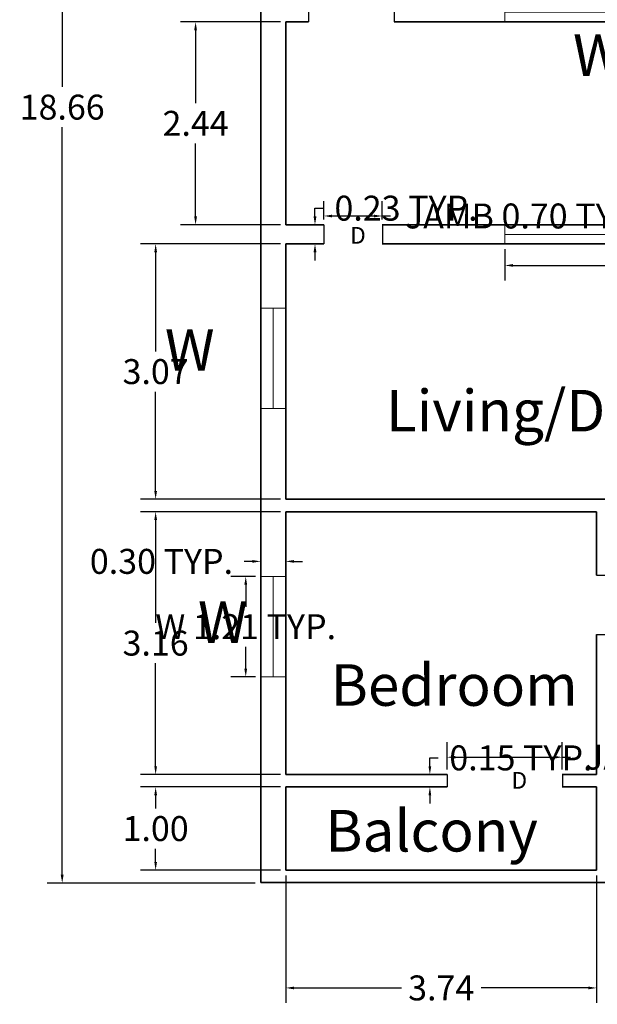
# Model space of a CAD drawing. Units: metres. Extents: x 11 to 49.6, y -23.3 to -0.8.
# Tile 1 of 5: x 11 to 17.9, y -23.3 to -11.5. Entities that reach past the tile are written whole.
import ezdxf

# ---------------------------------------------------------------- set-up
doc = ezdxf.new("R2010")
doc.units = ezdxf.units.M
doc.header["$MEASUREMENT"] = 0
for name, color, linetype, lineweight in [('A-ANNO-DIMS', 2, 'Continuous', 18), ('A-ANNO-IDEN', 3, 'Continuous', 18), ('A-AREA-IDEN', 7, 'Continuous', 18), ('A-DOOR', 3, 'Continuous', 25), ('A-GLAZ', 4, 'Continuous', 18), ('A-WALL', 7, 'Continuous', 35)]:
    doc.layers.add(name, color=color, linetype=linetype, lineweight=lineweight)
doc.styles.get("Standard").update_dxf_attribs({"font": 'arial.ttf'})
doc.dimstyles.get("Standard").update_dxf_attribs({"dimtxt": 0.3, "dimasz": 0.1, "dimexe": 0.18, "dimexo": 0.0625, "dimgap": 0.09, "dimtad": 0, "dimtih": 1, "dimtoh": 1, "dimzin": 0, "dimdsep": 46, "dimtxsty": 'Standard', "dimcen": 0.09, "dimadec": 0, "dimazin": 0, "dimtfac": 1, "dimtofl": 0, "dimtmove": 0, "dimatfit": 3, "dimfxl": 1, "dimtolj": 1, "dimtzin": 0, "dimarcsym": 0})

# ---------------------------------------------------------------- blocks, each defined once
blk = doc.blocks.new('*D2')
at = {"layer": 'A-ANNO-DIMS', "color": 0, "lineweight": -2, "transparency": 16777216}
for p, q in [((13.833, -3.189), (11.33, -3.189)), ((11.51, -3.289), (11.51, -12.277)), ((11.51, -21.752), (11.51, -12.764)), ((13.833, -21.852), (11.33, -21.852))]:
    blk.add_line(p, q, dxfattribs=at)
at = {"layer": 'A-ANNO-DIMS', "color": 0, "transparency": 16777216}
for points in [[(11.493, -3.289), (11.527, -3.289), (11.51, -3.189)], [(11.493, -21.752), (11.527, -21.752), (11.51, -21.852)]]:
    blk.add_solid(points, dxfattribs=at)
at = {"layer": 'Defpoints', "color": 0, "transparency": 16777216}
for p in [(13.896, -3.189), (11.51, -21.852), (13.895, -21.852)]:
    blk.add_point(p, dxfattribs=at)
at = {"layer": 'A-ANNO-DIMS', "color": 0, "transparency": 16777216, "insert": (11.51, -12.521), "char_height": 0.3, "attachment_point": 5}
blk.add_mtext('\\A1;18.66', dxfattribs=at)
blk = doc.blocks.new('*D11')
at = {"layer": 'A-ANNO-DIMS', "color": 0, "lineweight": -2, "transparency": 16777216}
for p, q in [((14.137, -11.496), (12.935, -11.496)), ((13.115, -11.596), (13.115, -12.475)), ((13.115, -13.836), (13.115, -12.957)), ((14.137, -13.936), (12.935, -13.936))]:
    blk.add_line(p, q, dxfattribs=at)
at = {"layer": 'A-ANNO-DIMS', "color": 0, "transparency": 16777216}
for points in [[(13.098, -11.596), (13.131, -11.596), (13.115, -11.496)], [(13.098, -13.836), (13.131, -13.836), (13.115, -13.936)]]:
    blk.add_solid(points, dxfattribs=at)
at = {"layer": 'Defpoints', "color": 0, "transparency": 16777216}
for p in [(14.199, -11.496), (13.115, -13.936), (14.199, -13.936)]:
    blk.add_point(p, dxfattribs=at)
at = {"layer": 'A-ANNO-DIMS', "color": 0, "transparency": 16777216, "insert": (13.115, -12.716), "char_height": 0.3, "attachment_point": 5}
blk.add_mtext('\\A1;2.44', dxfattribs=at)
blk = doc.blocks.new('WIN-1207-D300')
for p, q in [((0.3, 1.207), (0, 1.207)), ((0.15, 1.207), (0.15, 0)), ((0, 0), (0.3, 0))]:
    blk.add_line(p, q)
blk = doc.blocks.new('WIN-1724-D230')
for p, q in [((0, 0.23), (0, 0)), ((1.724, 0.23), (1.724, 0)), ((0, 0.115), (1.724, 0.115))]:
    blk.add_line(p, q)
blk = doc.blocks.new('DOOR-JAMB-704')
for p, q in [((0, 0.23), (0, 0)), ((0.704, 0.23), (0.704, 0))]:
    blk.add_line(p, q)
blk = doc.blocks.new('DOOR-JAMB-1386')
for p, q in [((0, 0.15), (0, 0)), ((1.386, 0.15), (1.386, 0))]:
    blk.add_line(p, q)
blk = doc.blocks.new('*D28')
at = {"layer": 'A-ANNO-DIMS', "color": 0, "lineweight": -2, "transparency": 16777216}
for p, q in [((13.837, -18.165), (13.538, -18.165)), ((13.718, -18.265), (13.718, -18.528)), ((13.718, -19.272), (13.718, -19.009)), ((13.837, -19.372), (13.538, -19.372))]:
    blk.add_line(p, q, dxfattribs=at)
at = {"layer": 'A-ANNO-DIMS', "color": 0, "transparency": 16777216}
for points in [[(13.701, -18.265), (13.735, -18.265), (13.718, -18.165)], [(13.701, -19.272), (13.735, -19.272), (13.718, -19.372)]]:
    blk.add_solid(points, dxfattribs=at)
at = {"layer": 'Defpoints', "color": 0, "transparency": 16777216}
for p in [(13.899, -18.165), (13.718, -19.372), (13.899, -19.372)]:
    blk.add_point(p, dxfattribs=at)
at = {"layer": 'A-ANNO-DIMS', "color": 0, "transparency": 16777216, "insert": (13.718, -18.768), "char_height": 0.3, "attachment_point": 5}
blk.add_mtext('\\A1;W 1.21 TYP.', dxfattribs=at)
blk = doc.blocks.new('*D29')
at = {"layer": 'A-ANNO-DIMS', "color": 0, "lineweight": -2, "transparency": 16777216}
for p, q in [((13.899, -18.102), (13.899, -17.803)), ((14.199, -18.102), (14.199, -17.803)), ((13.799, -17.983), (13.699, -17.983)), ((14.299, -17.983), (14.399, -17.983))]:
    blk.add_line(p, q, dxfattribs=at)
at = {"layer": 'A-ANNO-DIMS', "color": 0, "transparency": 16777216}
for points in [[(13.799, -17.967), (13.799, -18), (13.899, -17.983)], [(14.299, -17.967), (14.299, -18), (14.199, -17.983)]]:
    blk.add_solid(points, dxfattribs=at)
at = {"layer": 'Defpoints', "color": 0, "transparency": 16777216}
for p in [(13.899, -17.983), (13.899, -18.165), (14.199, -18.165)]:
    blk.add_point(p, dxfattribs=at)
at = {"layer": 'A-ANNO-DIMS', "color": 0, "transparency": 16777216, "insert": (12.704, -17.983), "char_height": 0.3, "attachment_point": 5}
blk.add_mtext('\\A1;0.30 TYP.', dxfattribs=at)
blk = doc.blocks.new('*D30')
at = {"layer": 'A-ANNO-DIMS', "color": 0, "lineweight": -2, "transparency": 16777216}
for p, q in [((16.834, -14.229), (16.834, -14.605)), ((18.558, -14.229), (18.558, -14.605)), ((16.934, -14.425), (18.458, -14.425)), ((18.558, -14.425), (18.658, -14.425))]:
    blk.add_line(p, q, dxfattribs=at)
at = {"layer": 'A-ANNO-DIMS', "color": 0, "transparency": 16777216}
for points in [[(16.934, -14.408), (16.934, -14.441), (16.834, -14.425)], [(18.458, -14.408), (18.458, -14.441), (18.558, -14.425)]]:
    blk.add_solid(points, dxfattribs=at)
at = {"layer": 'Defpoints', "color": 0, "transparency": 16777216}
for p in [(16.834, -14.166), (18.558, -14.166), (18.558, -14.425)]:
    blk.add_point(p, dxfattribs=at)
at = {"layer": 'A-ANNO-DIMS', "color": 0, "transparency": 16777216, "insert": (19.915, -14.425), "char_height": 0.3, "attachment_point": 5}
blk.add_mtext('\\A1;W 1.72 TYP.', dxfattribs=at)
blk = doc.blocks.new('*D42')
at = {"layer": 'A-ANNO-DIMS', "color": 0, "lineweight": -2, "transparency": 16777216}
for p, q in [((14.657, -13.874), (14.657, -13.65)), ((15.36, -13.874), (15.36, -13.65)), ((14.757, -13.83), (15.26, -13.83)), ((15.36, -13.83), (15.46, -13.83))]:
    blk.add_line(p, q, dxfattribs=at)
at = {"layer": 'A-ANNO-DIMS', "color": 0, "transparency": 16777216}
for points in [[(14.757, -13.814), (14.757, -13.847), (14.657, -13.83)], [(15.26, -13.814), (15.26, -13.847), (15.36, -13.83)]]:
    blk.add_solid(points, dxfattribs=at)
at = {"layer": 'Defpoints', "color": 0, "transparency": 16777216}
for p in [(15.36, -13.83), (14.657, -13.936), (15.36, -13.936)]:
    blk.add_point(p, dxfattribs=at)
at = {"layer": 'A-ANNO-DIMS', "color": 0, "transparency": 16777216, "insert": (17.075, -13.83), "char_height": 0.3, "attachment_point": 5}
blk.add_mtext('\\A1;JAMB 0.70 TYP.', dxfattribs=at)
blk = doc.blocks.new('*D43')
at = {"layer": 'A-ANNO-DIMS', "color": 0, "lineweight": -2, "transparency": 16777216}
for p, q in [((14.551, -13.836), (14.551, -13.736)), ((14.551, -13.736), (14.651, -13.736)), ((14.594, -13.936), (14.371, -13.936)), ((14.594, -14.166), (14.371, -14.166)), ((14.551, -14.266), (14.551, -14.366))]:
    blk.add_line(p, q, dxfattribs=at)
at = {"layer": 'A-ANNO-DIMS', "color": 0, "transparency": 16777216}
for points in [[(14.534, -13.836), (14.568, -13.836), (14.551, -13.936)], [(14.534, -14.266), (14.568, -14.266), (14.551, -14.166)]]:
    blk.add_solid(points, dxfattribs=at)
at = {"layer": 'Defpoints', "color": 0, "transparency": 16777216}
for p in [(14.551, -13.936), (14.657, -13.936), (14.657, -14.166)]:
    blk.add_point(p, dxfattribs=at)
at = {"layer": 'A-ANNO-DIMS', "color": 0, "transparency": 16777216, "insert": (15.646, -13.736), "char_height": 0.3, "attachment_point": 5}
blk.add_mtext('\\A1;0.23 TYP.', dxfattribs=at)
blk = doc.blocks.new('*D50')
at = {"layer": 'A-ANNO-DIMS', "color": 0, "lineweight": -2, "transparency": 16777216}
for p, q in [((16.141, -20.484), (16.141, -20.158)), ((17.526, -20.484), (17.526, -20.158)), ((16.241, -20.338), (17.426, -20.338)), ((17.526, -20.338), (17.626, -20.338))]:
    blk.add_line(p, q, dxfattribs=at)
at = {"layer": 'A-ANNO-DIMS', "color": 0, "transparency": 16777216}
for points in [[(16.241, -20.321), (16.241, -20.355), (16.141, -20.338)], [(17.426, -20.321), (17.426, -20.355), (17.526, -20.338)]]:
    blk.add_solid(points, dxfattribs=at)
at = {"layer": 'Defpoints', "color": 0, "transparency": 16777216}
for p in [(17.526, -20.338), (16.141, -20.546), (17.526, -20.546)]:
    blk.add_point(p, dxfattribs=at)
at = {"layer": 'A-ANNO-DIMS', "color": 0, "transparency": 16777216, "insert": (19.242, -20.338), "char_height": 0.3, "attachment_point": 5}
blk.add_mtext('\\A1;JAMB 1.39 TYP.', dxfattribs=at)
blk = doc.blocks.new('*D51')
at = {"layer": 'A-ANNO-DIMS', "color": 0, "lineweight": -2, "transparency": 16777216}
for p, q in [((15.933, -20.446), (15.933, -20.346)), ((15.933, -20.346), (16.033, -20.346)), ((16.078, -20.546), (15.753, -20.546)), ((16.078, -20.696), (15.753, -20.696)), ((15.933, -20.796), (15.933, -20.896))]:
    blk.add_line(p, q, dxfattribs=at)
at = {"layer": 'A-ANNO-DIMS', "color": 0, "transparency": 16777216}
for points in [[(15.916, -20.446), (15.949, -20.446), (15.933, -20.546)], [(15.916, -20.796), (15.949, -20.796), (15.933, -20.696)]]:
    blk.add_solid(points, dxfattribs=at)
at = {"layer": 'Defpoints', "color": 0, "transparency": 16777216}
for p in [(15.933, -20.546), (16.141, -20.546), (16.141, -20.696)]:
    blk.add_point(p, dxfattribs=at)
at = {"layer": 'A-ANNO-DIMS', "color": 0, "transparency": 16777216, "insert": (17.028, -20.346), "char_height": 0.3, "attachment_point": 5}
blk.add_mtext('\\A1;0.15 TYP.', dxfattribs=at)
blk = doc.blocks.new('*D65')
at = {"layer": 'A-ANNO-DIMS', "color": 0, "lineweight": -2, "transparency": 16777216}
for p, q in [((14.137, -14.166), (12.454, -14.166)), ((12.634, -14.266), (12.634, -15.458)), ((12.634, -17.136), (12.634, -15.944)), ((14.137, -17.236), (12.454, -17.236))]:
    blk.add_line(p, q, dxfattribs=at)
at = {"layer": 'A-ANNO-DIMS', "color": 0, "transparency": 16777216}
for points in [[(12.618, -14.266), (12.651, -14.266), (12.634, -14.166)], [(12.618, -17.136), (12.651, -17.136), (12.634, -17.236)]]:
    blk.add_solid(points, dxfattribs=at)
at = {"layer": 'Defpoints', "color": 0, "transparency": 16777216}
for p in [(14.199, -14.166), (12.634, -17.236), (14.199, -17.236)]:
    blk.add_point(p, dxfattribs=at)
at = {"layer": 'A-ANNO-DIMS', "color": 0, "transparency": 16777216, "insert": (12.634, -15.701), "char_height": 0.3, "attachment_point": 5}
blk.add_mtext('\\A1;3.07', dxfattribs=at)
blk = doc.blocks.new('*D66')
at = {"layer": 'A-ANNO-DIMS', "color": 0, "lineweight": -2, "transparency": 16777216}
for p, q in [((14.137, -17.386), (12.454, -17.386)), ((12.634, -17.486), (12.634, -18.723)), ((12.634, -20.446), (12.634, -19.209)), ((14.137, -20.546), (12.454, -20.546))]:
    blk.add_line(p, q, dxfattribs=at)
at = {"layer": 'A-ANNO-DIMS', "color": 0, "transparency": 16777216}
for points in [[(12.618, -17.486), (12.651, -17.486), (12.634, -17.386)], [(12.618, -20.446), (12.651, -20.446), (12.634, -20.546)]]:
    blk.add_solid(points, dxfattribs=at)
at = {"layer": 'Defpoints', "color": 0, "transparency": 16777216}
for p in [(14.199, -17.386), (12.634, -20.546), (14.199, -20.546)]:
    blk.add_point(p, dxfattribs=at)
at = {"layer": 'A-ANNO-DIMS', "color": 0, "transparency": 16777216, "insert": (12.634, -18.966), "char_height": 0.3, "attachment_point": 5}
blk.add_mtext('\\A1;3.16', dxfattribs=at)
blk = doc.blocks.new('*D67')
at = {"layer": 'A-ANNO-DIMS', "color": 0, "lineweight": -2, "transparency": 16777216}
for p, q in [((14.137, -20.696), (12.454, -20.696)), ((12.634, -20.796), (12.634, -20.953)), ((12.634, -21.596), (12.634, -21.439)), ((14.137, -21.696), (12.454, -21.696))]:
    blk.add_line(p, q, dxfattribs=at)
at = {"layer": 'A-ANNO-DIMS', "color": 0, "transparency": 16777216}
for points in [[(12.618, -20.796), (12.651, -20.796), (12.634, -20.696)], [(12.618, -21.596), (12.651, -21.596), (12.634, -21.696)]]:
    blk.add_solid(points, dxfattribs=at)
at = {"layer": 'Defpoints', "color": 0, "transparency": 16777216}
for p in [(14.199, -20.696), (12.634, -21.696), (14.199, -21.696)]:
    blk.add_point(p, dxfattribs=at)
at = {"layer": 'A-ANNO-DIMS', "color": 0, "transparency": 16777216, "insert": (12.634, -21.196), "char_height": 0.3, "attachment_point": 5}
blk.add_mtext('\\A1;1.00', dxfattribs=at)
blk = doc.blocks.new('*D68')
at = {"layer": 'A-ANNO-DIMS', "color": 0, "lineweight": -2, "transparency": 16777216}
for p, q in [((14.199, -21.759), (14.199, -23.292)), ((17.939, -21.759), (17.939, -23.292)), ((14.299, -23.112), (15.59, -23.112)), ((17.839, -23.112), (16.548, -23.112))]:
    blk.add_line(p, q, dxfattribs=at)
at = {"layer": 'A-ANNO-DIMS', "color": 0, "transparency": 16777216}
for points in [[(14.299, -23.096), (14.299, -23.129), (14.199, -23.112)], [(17.839, -23.096), (17.839, -23.129), (17.939, -23.112)]]:
    blk.add_solid(points, dxfattribs=at)
at = {"layer": 'Defpoints', "color": 0, "transparency": 16777216}
for p in [(14.199, -21.696), (17.939, -21.696), (17.939, -23.112)]:
    blk.add_point(p, dxfattribs=at)
at = {"layer": 'A-ANNO-DIMS', "color": 0, "transparency": 16777216, "insert": (16.069, -23.112), "char_height": 0.3, "attachment_point": 5}
blk.add_mtext('\\A1;3.74', dxfattribs=at)

msp = doc.modelspace()

# ---------------------------------------------------------------- linework, layer by layer
at = {"layer": 'A-DOOR'}
for p, q in [((14.474, -11.266), (14.474, -11.496)), ((15.505, -11.266), (15.505, -11.496)), ((17.939, -18.147), (18.089, -18.147)), ((17.939, -18.863), (18.089, -18.863))]:
    msp.add_line(p, q, dxfattribs=at)
at = {"layer": 'A-WALL'}
for p, q in [((13.899, -3.186), (13.899, -14.166)), ((14.199, -11.496), (14.474, -11.496)), ((14.199, -11.496), (14.199, -13.936)), ((14.199, -11.496), (14.474, -11.496)), ((14.199, -13.936), (14.199, -11.496)), ((14.199, -11.496), (14.199, -13.936)), ((15.505, -11.496), (26.444, -11.496)), ((15.505, -11.496), (26.444, -11.496)), ((14.199, -13.936), (14.657, -13.936)), ((14.199, -13.936), (14.657, -13.936)), ((15.36, -13.936), (26.068, -13.936)), ((15.36, -13.936), (26.068, -13.936)), ((13.899, -14.166), (13.899, -21.846)), ((14.199, -14.166), (14.657, -14.166)), ((14.199, -14.166), (14.199, -17.236)), ((15.36, -14.166), (19.459, -14.166)), ((15.36, -14.166), (19.459, -14.166)), ((14.199, -17.236), (18.089, -17.236)), ((14.199, -17.386), (17.939, -17.386)), ((14.199, -17.386), (14.199, -20.546)), ((17.939, -18.147), (17.939, -17.386)), ((17.939, -20.546), (17.939, -18.863)), ((14.199, -20.546), (16.141, -20.546)), ((17.526, -20.546), (17.939, -20.546)), ((14.199, -20.696), (16.141, -20.696)), ((14.199, -20.696), (14.199, -21.696)), ((17.526, -20.696), (17.939, -20.696)), ((17.939, -21.696), (17.939, -20.696)), ((14.199, -21.696), (17.939, -21.696)), ((13.899, -21.846), (25.48, -21.846))]:
    msp.add_line(p, q, dxfattribs=at)

# ---------------------------------------------------------------- block references
at = {"layer": 'A-DOOR'}
for name, p in [('DOOR-JAMB-704', (14.657, -14.166)), ('DOOR-JAMB-1386', (16.141, -20.696))]:
    msp.add_blockref(name, p, dxfattribs=at)
at = {"layer": 'A-GLAZ'}
for p in [(16.834, -11.496), (16.834, -14.166)]:
    msp.add_blockref('WIN-1724-D230', p, dxfattribs=at)
at = {"layer": 'A-GLAZ', "rotation": 180}
for p in [(14.199, -14.939), (14.199, -18.165)]:
    msp.add_blockref('WIN-1207-D300', p, dxfattribs=at)

# ---------------------------------------------------------------- texts
at = {"layer": 'A-ANNO-IDEN', "attachment_point": 1}
for s, width, insert, char_height in [('W', 1.41386, (17.654, -11.645), 0.5), ('D', 0.77129, (14.974, -13.963), 0.2), ('W', 1.41386, (12.745, -15.191), 0.5), ('W', 1.41386, (13.143, -18.463), 0.5), ('D', 0.77129, (16.915, -20.516), 0.2), ('D', 0.77129, (16.915, -20.516), 0.2)]:
    msp.add_mtext_dynamic_manual_height_columns(s, width=width, gutter_width=0.5, heights=[0], dxfattribs=dict(at, insert=insert, char_height=char_height))
at = {"layer": 'A-AREA-IDEN', "char_height": 0.5, "attachment_point": 7}
for s, insert in [('Living/Dining', (15.404, -16.421)), ('Bedroom', (14.739, -19.72)), ('Balcony', (14.674, -21.472))]:
    msp.add_mtext_dynamic_manual_height_columns(s, width=2.63335, gutter_width=1, heights=[0], dxfattribs=dict(at, insert=insert))

# ---------------------------------------------------------------- dimensions: what is measured, and where the dimension line sits
at = {"layer": 'A-ANNO-DIMS'}
for base, p1, p2, override, picture, middle in [((11.51, -21.852), (13.896, -3.189), (13.895, -21.852), {"dimclrd": 0, "dimclre": 0, "dimclrt": 0}, '*D2', (11.51, -12.521)), ((13.115, -13.936), (14.199, -11.496), (14.199, -13.936), {"dimclrd": 0, "dimclre": 0, "dimclrt": 0}, '*D11', (13.115, -12.716)), ((12.634, -17.236), (14.199, -14.166), (14.199, -17.236), {"dimdec": 2, "dimlfac": 1, "dimrnd": 0, "dimzin": 0, "dimdsep": 46, "dimlunit": 2}, '*D65', (12.634, -15.701)), ((12.634, -20.546), (14.199, -17.386), (14.199, -20.546), {"dimdec": 2, "dimlfac": 1, "dimrnd": 0, "dimzin": 0, "dimdsep": 46, "dimlunit": 2}, '*D66', (12.634, -18.966)), ((12.634, -21.696), (14.199, -20.696), (14.199, -21.696), {"dimdec": 2, "dimlfac": 1, "dimrnd": 0, "dimzin": 0, "dimdsep": 46, "dimlunit": 2}, '*D67', (12.634, -21.196))]:
    dim = msp.add_linear_dim(base=base, p1=p1, p2=p2, angle=90, dimstyle='Standard', override=override, dxfattribs=at)
    dim.commit()
    dim.dimension.update_dxf_attribs({"geometry": picture, "text_midpoint": middle})
for base, p1, p2, text, picture, middle in [((15.36, -13.83), (14.657, -13.936), (15.36, -13.936), 'JAMB <> TYP.', '*D42', (17.075, -13.83)), ((18.558, -14.425), (16.834, -14.166), (18.558, -14.166), 'W <> TYP.', '*D30', (19.915, -14.425)), ((17.5264, -20.3382), (16.1406, -20.546), (17.5264, -20.546), 'JAMB <> TYP.', '*D50', (19.2415, -20.3382))]:
    dim = msp.add_linear_dim(base=base, p1=p1, p2=p2, text=text, dimstyle='Standard', override={"dimdec": 2, "dimlfac": 1, "dimrnd": 0, "dimzin": 0, "dimdsep": 46, "dimlunit": 2}, dxfattribs=at)
    dim.commit()
    dim.dimension.update_dxf_attribs({"geometry": picture, "text_midpoint": middle})
for base, p1, p2, angle, text, picture, middle in [((14.551, -13.936), (14.657, -14.166), (14.657, -13.936), 90, '<> TYP.', '*D43', (15.646, -13.736)), ((13.899, -17.983), (14.199, -18.165), (13.899, -18.165), 180, '<> TYP.', '*D29', (12.704, -17.983)), ((13.718, -19.372), (13.899, -18.165), (13.899, -19.372), 270, 'W <> TYP.', '*D28', (13.718, -18.768)), ((15.933, -20.546), (16.141, -20.696), (16.141, -20.546), 90, '<> TYP.', '*D51', (17.028, -20.346))]:
    dim = msp.add_linear_dim(base=base, p1=p1, p2=p2, angle=angle, text=text, dimstyle='Standard', override={"dimdec": 2, "dimlfac": 1, "dimrnd": 0, "dimzin": 0, "dimdsep": 46, "dimlunit": 2}, dxfattribs=at)
    dim.commit()
    dim.dimension.update_dxf_attribs({"geometry": picture, "text_midpoint": middle})
dim = msp.add_linear_dim(base=(17.939, -23.112), p1=(14.199, -21.696), p2=(17.939, -21.696), dimstyle='Standard', override={"dimdec": 2, "dimlfac": 1, "dimrnd": 0, "dimzin": 0, "dimdsep": 46, "dimlunit": 2}, dxfattribs=at)
dim.commit()
dim.dimension.update_dxf_attribs({"geometry": '*D68', "text_midpoint": (16.069, -23.112)})

doc.saveas('drawing.dxf')
